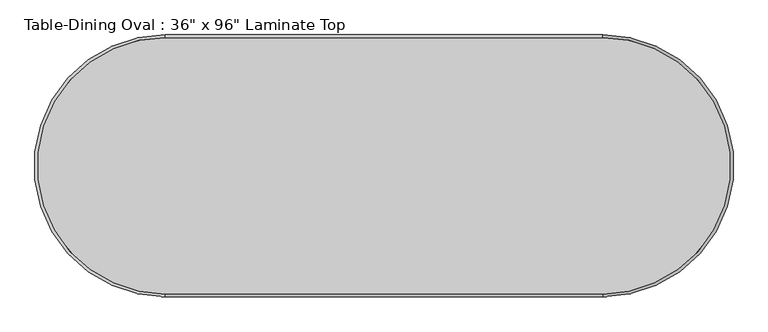
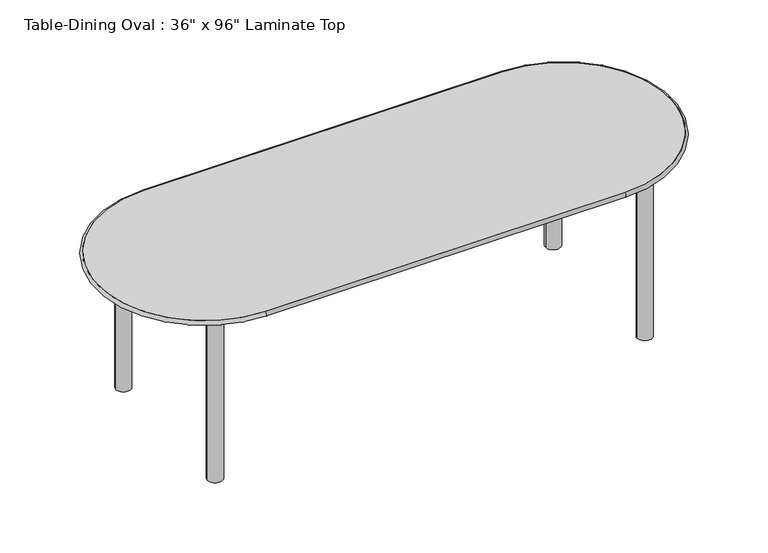
"""IFC4 building model written with IfcOpenShell, lengths in millimetres: furniture geometry."""

from ifc_helpers import new_model, si_unit, point, frame, frame_2d, origin, origin_with_axes, place, context, project, spatial, polyline, circle_curve, ellipse_curve, trimmed, segment, composite_curve, outline, extrude, source, transform, mapped, element, save
from ifc_brep_helpers import plane_surface, cylinder_surface, revolved_surface, advanced_brep


def furniture_e05f6f82(model_context):
    return source(origin(), model_context, "Body", "SolidModel", [
        advanced_brep(
        [(-1163.8196721, -805.7733607, 762.0), (-1163.8196721, -805.7733607, 742.95), (360.1803279, -805.7733607, 742.95), (360.1803279, -805.7733607, 762.0), (360.1803279, 89.5766393, 762.0), (360.1803279, 89.5766393, 742.95), (-1163.8196721, 89.5766393, 742.95), (-1163.8196721, 89.5766393, 762.0)],
        [
            (0, 1, circle_curve(frame((-1163.8196721, -805.7733607, 752.475), z_axis=(1.0, 0.0, 0.0), x_axis=(0.0, 1.0, 0.0)), 9.525)),
            (1, 2),
            (2, 3, circle_curve(frame((360.1803279, -805.7733607, 752.475), z_axis=(-1.0, 0.0, 0.0), x_axis=(0.0, 1.0, 0.0)), 9.525)),
            (3, 0),
            (1, 0),
            (3, 2),
            (4, 3, circle_curve(frame((360.1803279, -358.0983607, 762.0), z_axis=(0.0, 0.0, -1.0), x_axis=(0.0, -1.0, 0.0)), 447.675)),
            (2, 5, circle_curve(frame((360.1803279, -358.0983607, 742.95), z_axis=(0.0, 0.0, 1.0), x_axis=(0.0, -1.0, 0.0)), 447.675)),
            (5, 4, circle_curve(frame((360.1803279, 89.5766393, 752.475), z_axis=(1.0, 0.0, 0.0), x_axis=(0.0, -1.0, 0.0)), 9.525)),
            (4, 5),
            (5, 6),
            (6, 7, circle_curve(frame((-1163.8196721, 89.5766393, 752.475), z_axis=(1.0, 0.0, 0.0), x_axis=(0.0, -1.0, 0.0)), 9.525)),
            (7, 4),
            (7, 6),
            (0, 7, circle_curve(frame((-1163.8196721, -358.0983607, 762.0), z_axis=(0.0, 0.0, -1.0), x_axis=(0.0, 1.0, 0.0)), 447.675)),
            (6, 1, circle_curve(frame((-1163.8196721, -358.0983607, 742.95), z_axis=(0.0, 0.0, 1.0), x_axis=(0.0, 1.0, 0.0)), 447.675)),
        ],
        [
            cylinder_surface(frame((-1163.8196721, -805.7733607, 752.475), z_axis=(-1.0, 0.0, 0.0), x_axis=(0.0, 1.0, 0.0)), 9.525),
            plane_surface(frame((-1163.8196721, -805.7733607, 762.0), z_axis=(0.0, 1.0, 0.0), x_axis=(1.0, 0.0, 0.0))),
            revolved_surface(trimmed(ellipse_curve(frame((360.1803279, -805.7733607, 752.475), z_axis=(-1.0, 0.0, 0.0), x_axis=(0.0, 1.0, 0.0)), 9.525, 9.525), [point((360.1803279, -805.7733607, 742.95))], [point((360.1803279, -805.7733607, 762.0))], True, "CARTESIAN"), (360.1803279, -358.0983607, 0.0), (0.0, 0.0, 1.0)),
            revolved_surface(polyline([(360.1803279, -805.7733607, 762.0), (360.1803279, -805.7733607, 742.95)]), (360.1803279, -358.0983607, 0.0), (0.0, 0.0, 1.0)),
            cylinder_surface(frame((360.1803279, 89.5766393, 752.475), z_axis=(1.0, 0.0, 0.0), x_axis=(0.0, -1.0, 0.0)), 9.525),
            plane_surface(frame((360.1803279, 89.5766393, 762.0), z_axis=(0.0, -1.0, 0.0), x_axis=(-1.0, 0.0, 0.0))),
            revolved_surface(trimmed(ellipse_curve(frame((-1163.8196721, 89.5766393, 752.475), z_axis=(1.0, 0.0, 0.0), x_axis=(0.0, -1.0, 0.0)), 9.525, 9.525), [point((-1163.8196721, 89.5766393, 742.95))], [point((-1163.8196721, 89.5766393, 762.0))], True, "CARTESIAN"), (-1163.8196721, -358.0983607, 0.0), (0.0, 0.0, 1.0)),
            revolved_surface(polyline([(-1163.8196721, 89.57663930000001, 762.0), (-1163.8196721, 89.57663930000001, 742.95)]), (-1163.8196721, -358.0983607, 0.0), (0.0, 0.0, 1.0)),
        ],
        [
            (0, [[1, 2, 3, 4]]),
            (1, [[5, -4, 6, -2]]),
            (2, [[7, -3, 8, 9]]),
            (3, [[-8, -6, -7, 10]]),
            (4, [[-9, 11, 12, 13]]),
            (5, [[-10, -13, 14, -11]]),
            (6, [[15, -12, 16, -1]]),
            (7, [[-16, -14, -15, -5]]),
        ],
    ),
        extrude(outline(composite_curve([segment(trimmed(circle_curve(frame_2d((-1313.0446721, -21.5483607)), 31.75), [point((-1344.7946721, -21.5483607))], [point((-1281.2946721, -21.5483607))], False, "CARTESIAN"), True, "CONTINUOUS"), segment(trimmed(circle_curve(frame_2d((-1313.0446721, -21.5483607)), 31.75), [point((-1281.2946721, -21.5483607))], [point((-1344.7946721, -21.5483607))], False, "CARTESIAN"), True, "CONTINUOUS")], self_intersect=False)), origin_with_axes(), (0.0, 0.0, 1.0), 742.95),
        extrude(outline(composite_curve([segment(trimmed(circle_curve(frame_2d((-1313.0446721, -694.6483607)), 31.75), [point((-1344.7946721, -694.6483607))], [point((-1281.2946721, -694.6483607))], False, "CARTESIAN"), True, "CONTINUOUS"), segment(trimmed(circle_curve(frame_2d((-1313.0446721, -694.6483607)), 31.75), [point((-1281.2946721, -694.6483607))], [point((-1344.7946721, -694.6483607))], False, "CARTESIAN"), True, "CONTINUOUS")], self_intersect=False)), origin_with_axes(), (0.0, 0.0, 1.0), 742.95),
        extrude(outline(composite_curve([segment(trimmed(circle_curve(frame_2d((509.4053279, -21.5483607)), 31.75), [point((477.6553279, -21.5483607))], [point((541.1553279, -21.5483607))], False, "CARTESIAN"), True, "CONTINUOUS"), segment(trimmed(circle_curve(frame_2d((509.4053279, -21.5483607)), 31.75), [point((541.1553279, -21.5483607))], [point((477.6553279, -21.5483607))], False, "CARTESIAN"), True, "CONTINUOUS")], self_intersect=False)), origin_with_axes(), (0.0, 0.0, 1.0), 742.95),
        extrude(outline(composite_curve([segment(trimmed(circle_curve(frame_2d((509.4053279, -694.6483607)), 31.75), [point((477.6553279, -694.6483607))], [point((541.1553279, -694.6483607))], False, "CARTESIAN"), True, "CONTINUOUS"), segment(trimmed(circle_curve(frame_2d((509.4053279, -694.6483607)), 31.75), [point((541.1553279, -694.6483607))], [point((477.6553279, -694.6483607))], False, "CARTESIAN"), True, "CONTINUOUS")], self_intersect=False)), origin_with_axes(), (0.0, 0.0, 1.0), 742.95),
        extrude(outline(polyline([(528.4553279, -2.4983607), (528.4553279, -713.6983607), (-1332.0946721, -713.6983607), (-1332.0946721, -2.4983607), (528.4553279, -2.4983607)]), holes=[polyline([(509.4053279, -21.5483607), (-1313.0446721, -21.5483607), (-1313.0446721, -694.6483607), (509.4053279, -694.6483607), (509.4053279, -21.5483607)])]), frame((0.0, 0.0, 692.15), z_axis=(0.0, 0.0, 1.0), x_axis=(1.0, 0.0, 0.0)), (0.0, 0.0, 1.0), 50.8),
        extrude(outline(composite_curve([segment(polyline([(-1163.8196721, 89.5766393), (360.1803279, 89.5766393)]), True, "CONTINUOUS"), segment(trimmed(circle_curve(frame_2d((360.1803279, -358.0983607)), 447.675), [point((360.1803279, 89.5766393))], [point((807.8553279, -358.0983607))], False, "CARTESIAN"), True, "CONTINUOUS"), segment(trimmed(circle_curve(frame_2d((360.1803279, -358.0983607)), 447.675), [point((807.8553279, -358.0983607))], [point((360.1803279, -805.7733607))], False, "CARTESIAN"), True, "CONTINUOUS"), segment(polyline([(360.1803279, -805.7733607), (-1163.8196721, -805.7733607)]), True, "CONTINUOUS"), segment(trimmed(circle_curve(frame_2d((-1163.8196721, -358.0983607)), 447.675), [point((-1163.8196721, -805.7733607))], [point((-1611.4946721, -358.0983607))], False, "CARTESIAN"), True, "CONTINUOUS"), segment(trimmed(circle_curve(frame_2d((-1163.8196721, -358.0983607)), 447.675), [point((-1611.4946721, -358.0983607))], [point((-1163.8196721, 89.5766393))], False, "CARTESIAN"), True, "CONTINUOUS")], self_intersect=False)), frame((0.0, 0.0, 742.95), z_axis=(0.0, 0.0, 1.0), x_axis=(1.0, 0.0, 0.0)), (0.0, 0.0, 1.0), 19.05),
    ])


if __name__ == "__main__":
    model = new_model("IFC4")
    model_context = context("Model", 3, world=origin())
    ifc_project = project(units=[si_unit("LENGTHUNIT", "METRE", prefix="MILLI")], contexts=[model_context])
    site = spatial("IfcSite", under=ifc_project)
    building = spatial("IfcBuilding", under=site)
    placement = place(None, origin())
    furniture_shape = furniture_e05f6f82(model_context)
    element("IfcFurniture", 1, ObjectType="Table-Dining Oval : 36\" x 96\" Laminate Top", at=placement, inside=building, context=model_context, shape_type="MappedRepresentation", body=[
        mapped(furniture_shape, transform((0.0, 0.0, 0.0), x_axis=(1.0, 0.0, 0.0), y_axis=(0.0, 1.0, 0.0), z_axis=(0.0, 0.0, 1.0))),
    ])
    save(model, "model.ifc")

# Revit data of these elements
# Type "Table-Dining Oval : 36\" x 96\" Laminate Top"
#   Assembly Code = "E2020200"
#   Length = 8' - 0"
#   Width = 3' - 0"
#   Base Material = Metal - Bronze, Light Brush
#   Top Material = Laminate, Ivory, Matte
#   Default Elevation = 0
#   Description = (empty or 0)
# Element 1 (IfcFurniture, "Table-Dining Oval : 36\" x 96\" Laminate Top")
#   Materials on its faces: "Metal - Bronze, Light Brush", "Glass - Clear, Grey", "Laminate, Ivory, Matte"
# Materials
#   "Metal - Bronze, Light Brush": class "Metal", colour RGB 113 80 70, transparency 0
#   "Laminate, Ivory, Matte": class "Plastic", colour RGB 247 247 239, transparency 0, Description = "Plastic Laminate - Ivory, Matte", Cost = 0
#   "Glass - Clear, Grey": class "Glass", colour RGB 252 255 255, transparency 0.64
